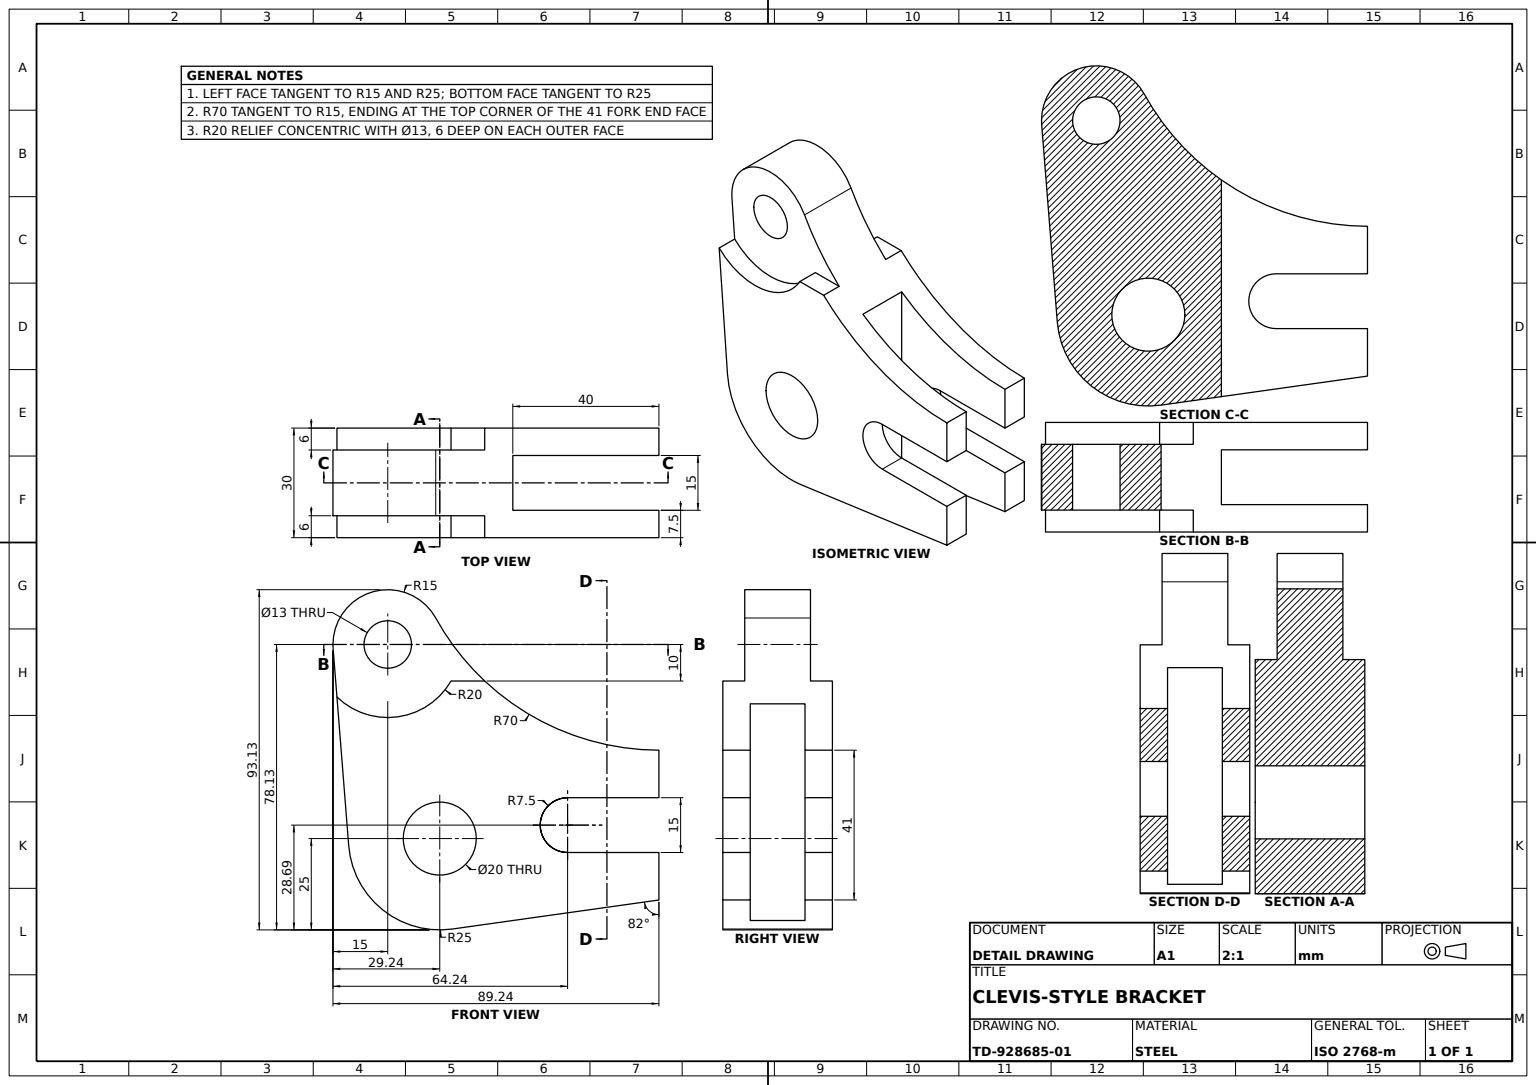
SolidWorks part; units mm, degrees
material "Plain Carbon Steel"
ref_plane "Front Plane" through (0, 0, 0) normal (0, 0, 1) x (1, 0, 0)
ref_plane "Top Plane" through (0, 0, 0) normal (0, 1, 0) x (1, 0, 0)
ref_plane "Right Plane" through (0, 0, 0) normal (1, 0, 0) x (0, 0, -1)
sketch "Bracket Profile Sketch" plane through (0, 0, 0) normal (1, 0, 0) x (0, 0, -1)
  line L0 (-24.9221, -1.9721) -> (-29.1883, 51.9427)
  line L2 (60, 24.1868) -> (60, 11.1868)
  line L3 (60, -16.8132) -> (3.4793, -24.7567)
  line L4 (0, 0) -> (-14.235, 53.1259) construction
  line L5 (60, 11.1868) -> (35, 11.1868)
  line L8 (35, -3.8132) -> (60, -3.8132)
  line L9 (60, -3.8132) -> (60, -16.8132)
  circle A0 centre (0, 0) radius 10
  arc A1 (-24.9221, -1.9721) -> (3.4793, -24.7567) centre (0, 0) ccw
  arc A2 (-29.1883, 51.9427) -> (-1.1013, 60.3719) centre (-14.235, 53.1259) cw
  arc A3 (-1.1013, 60.3719) -> (60, 24.1868) centre (60.1896, 94.1865) ccw
  circle A4 centre (-14.235, 53.1259) radius 6.5
  arc A6 (35, 11.1868) -> (35, -3.8132) centre (35, 3.6868) ccw
  dimension "D1" = 20
  dimension "D2" = 50
  dimension "D3" = 15
  dimension "D6" = 70
  dimension "D9" = 13
  dimension "D4" = 15
  dimension "D5" = 55
  dimension "D7" = 60
  dimension "D8" = 41
  dimension "D10" = 8
  dimension "D11" = 25
  dimension "D12" = 15
  dimension "D13" = 13
extrude "Bracket Body 30 Thick" add sketch "Bracket Profile Sketch" along normal mid plane 30
sketch "Side Step Sketch" plane through (15, 0, 0) normal (1, 0, 0) x (0, 0, -1)
  line L0 (-29.1883, 51.9427) -> (-24.9221, -1.9721) construction
  line L1 (3.0855, 43.1259) -> (12.3062, 43.1259)
  line L2 (-29.1883, 51.9427) -> (-28.1448, 38.7552)
  arc A0 (-28.1448, 38.7552) -> (3.0855, 43.1259) centre (-14.235, 53.1259) ccw
  arc A1 (-1.1013, 60.3719) -> (60, 24.1868) centre (60.1896, 94.1865) ccw construction
  arc A2 (-1.1013, 60.3719) -> (-29.1883, 51.9427) centre (-14.235, 53.1259) ccw construction
  arc A3 (-1.1013, 60.3719) -> (12.3062, 43.1259) centre (60.1896, 94.1865) ccw
  arc A4 (-1.1013, 60.3719) -> (-29.1883, 51.9427) centre (-14.235, 53.1259) ccw
  dimension "D1" = 20
  dimension "D2" = 10
extrude "Side Step Cut 20x10x6" cut sketch "Side Step Sketch" against normal blind 6
mirror "Side Step Cut Mirror" about plane through (0, 0, 0) normal (1, 0, 0) of "Side Step Cut 20x10x6"
sketch "Fork Slot Sketch" plane through (0, 0, 0) normal (0, 1, 0) x (1, 0, 0)
  line L0 (15, 60) -> (-15, 60) construction
  line L1 (-7.5, 60) -> (7.5, 60)
  line L2 (-7.5, 60) -> (-7.5, 20)
  line L3 (-7.5, 20) -> (7.5, 20)
  line L4 (7.5, 60) -> (7.5, 20)
  line L5 (0, 60) -> (0, 0) construction
  dimension "D1" = 40
  dimension "D2" = 15
extrude "Forked Slot 15 Wide" cut sketch "Fork Slot Sketch" along normal through all both and the other way through all
